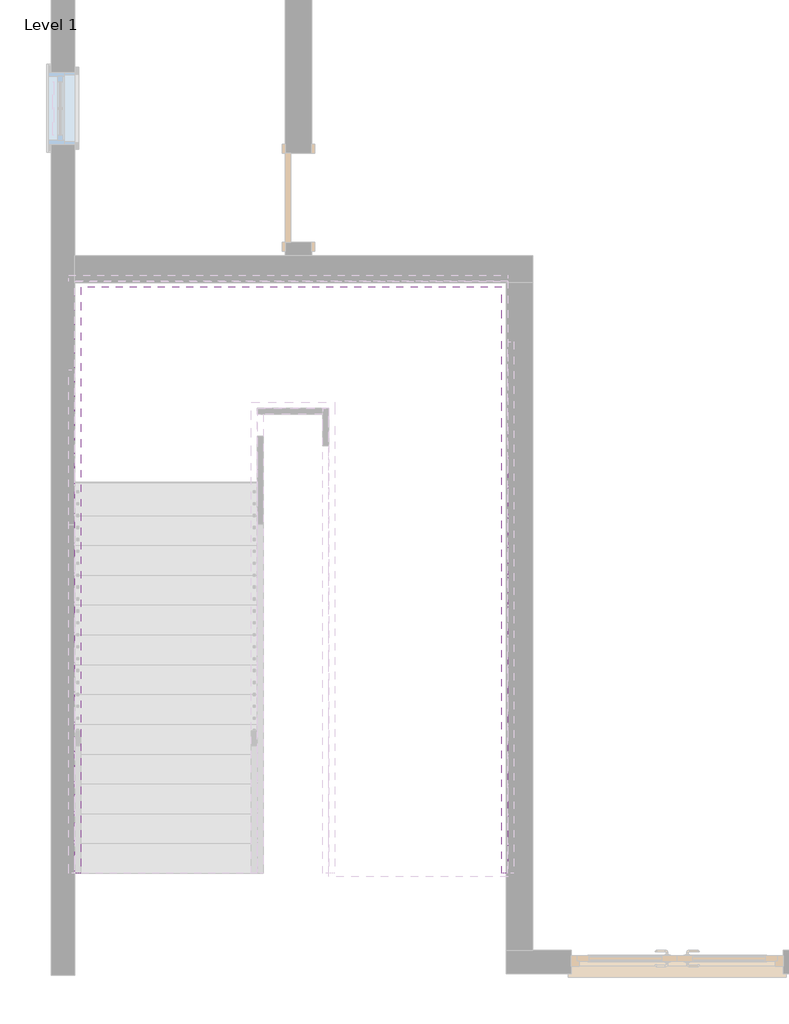
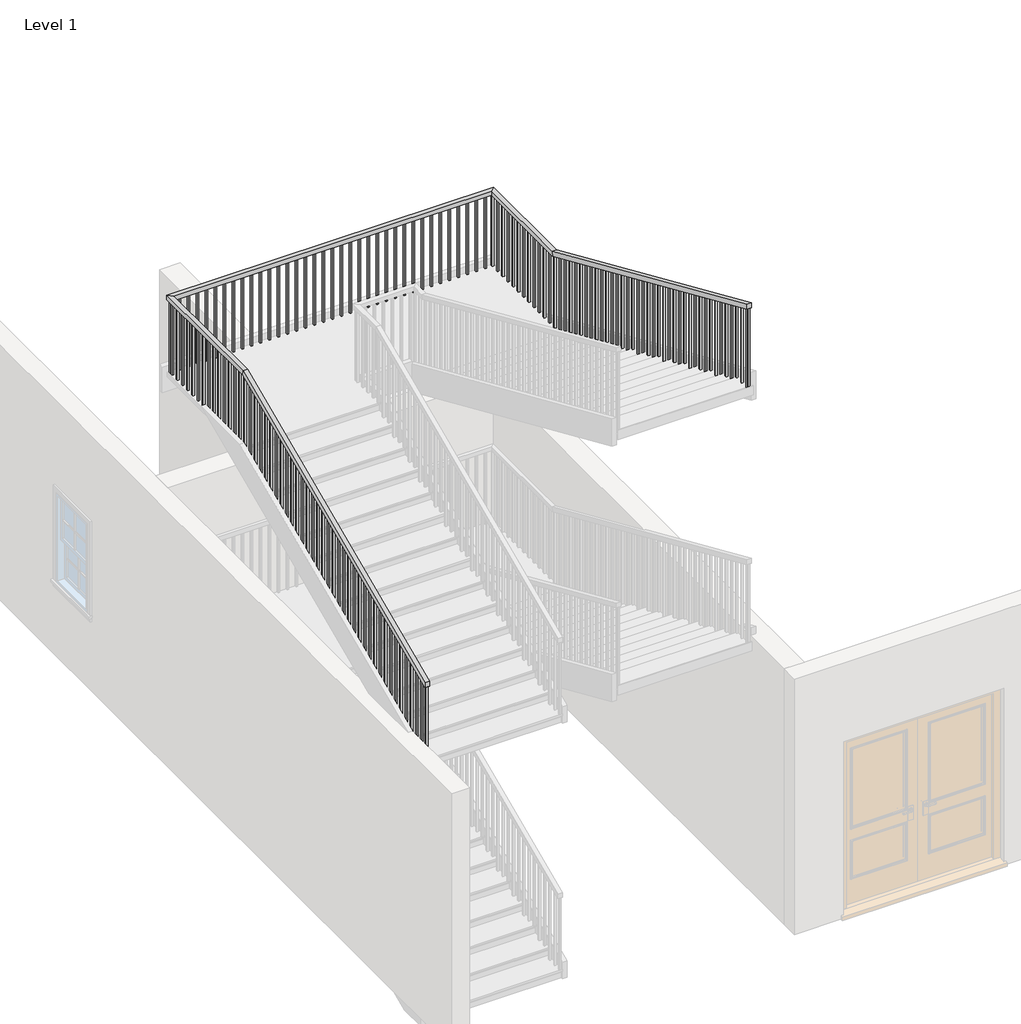
# One storey, part 5 of 6: 1 railing.
"""IFC4 building model written with IfcOpenShell, lengths in millimetres."""

from ifc_helpers import new_model, si_unit, frame, origin, place, context, project, spatial, polyline, outline, extrude, faceted_brep, element, save

model = new_model("IFC4")

# Units and contexts
model_context = context("Model", 3, world=origin())
ifc_project = project(units=[si_unit("LENGTHUNIT", "METRE", prefix="MILLI")], contexts=[model_context])

# Site, building, storey
site = spatial("IfcSite", under=ifc_project)
building = spatial("IfcBuilding", under=site)
storey = spatial("IfcBuildingStorey", under=building, Name="Level 1", Elevation=0.0)

# Railing
placement = place(None, origin())
element("IfcRailing", 1, ObjectType="Handrail - Rectangular", at=placement, inside=storey, context=model_context, shape_type="SolidModel", body=[
    faceted_brep([(-7554.4415084, -6973.0610642, 3769.36), (-7554.4415084, -6973.0610642, 3713.8599828), (-7503.6415084, -6973.0610642, 3713.8599828), (-7503.6415084, -6973.0610642, 3769.36), (-7554.4415084, -3417.0610642, 5334.0), (-7554.4415084, -3406.3792071, 5283.2), (-7503.6415084, -3406.3792071, 5283.2), (-7503.6415084, -3417.0610642, 5334.0), (-7554.4415084, -1928.4217109, 5334.0), (-7554.4415084, -1928.4217109, 5283.2), (-7503.6415084, -1979.2217109, 5283.2), (-7503.6415084, -1979.2217109, 5334.0), (-3866.3290366, -1928.4217109, 5334.0), (-3866.3290366, -1928.4217109, 5283.2), (-3917.1290366, -1979.2217109, 5283.2), (-3917.1290366, -1979.2217109, 5334.0), (-3866.3290366, -3163.0610642, 5334.0), (-3866.3290366, -3173.7429214, 5283.2), (-3917.1290366, -3173.7429214, 5283.2), (-3917.1290366, -3163.0610642, 5334.0), (-3866.3290366, -6973.0610642, 7010.4), (-3917.1290366, -6973.0610642, 7010.4), (-3917.1290366, -6973.0610642, 6954.8999828), (-3866.3290366, -6973.0610642, 6954.8999828)], [[[0, 1, 2, 3]], [[1, 0, 4, 5]], [[2, 1, 5, 6]], [[3, 2, 6, 7]], [[0, 3, 7, 4]], [[5, 4, 8, 9]], [[6, 5, 9, 10]], [[7, 6, 10, 11]], [[4, 7, 11, 8]], [[9, 8, 12, 13]], [[10, 9, 13, 14]], [[11, 10, 14, 15]], [[8, 11, 15, 12]], [[13, 12, 16, 17]], [[14, 13, 17, 18]], [[15, 14, 18, 19]], [[12, 15, 19, 16]], [[20, 21, 22, 23]], [[17, 16, 20, 23]], [[18, 17, 23, 22]], [[19, 18, 22, 21]], [[16, 19, 21, 20]]]),
    extrude(outline(polyline([(-6922.6967109, 6932.7396674), (-6922.6967109, 5984.24), (-6941.7467109, 5984.24), (-6941.7467109, 6941.1216674), (-6922.6967109, 6932.7396674)])), frame((-3901.2540366, 0.0, 0.0), z_axis=(1.0, 0.0, 0.0), x_axis=(0.0, 1.0, 0.0)), (0.0, 0.0, 1.0), 19.05),
    extrude(outline(polyline([(-6821.0967109, 6888.0356674), (-6821.0967109, 5984.24), (-6840.1467109, 5984.24), (-6840.1467109, 6896.4176674), (-6821.0967109, 6888.0356674)])), frame((-3901.2540366, 0.0, 0.0), z_axis=(1.0, 0.0, 0.0), x_axis=(0.0, 1.0, 0.0)), (0.0, 0.0, 1.0), 19.05),
    extrude(outline(polyline([(-6719.4967109, 6843.3316674), (-6719.4967109, 5984.24), (-6738.5467109, 5984.24), (-6738.5467109, 6851.7136674), (-6719.4967109, 6843.3316674)])), frame((-3901.2540366, 0.0, 0.0), z_axis=(1.0, 0.0, 0.0), x_axis=(0.0, 1.0, 0.0)), (0.0, 0.0, 1.0), 19.05),
    extrude(outline(polyline([(-6617.8967109, 6798.6276674), (-6617.8967109, 5872.48), (-6636.9467109, 5872.48), (-6636.9467109, 6807.0096674), (-6617.8967109, 6798.6276674)])), frame((-3901.2540366, 0.0, 0.0), z_axis=(1.0, 0.0, 0.0), x_axis=(0.0, 1.0, 0.0)), (0.0, 0.0, 1.0), 19.05),
    extrude(outline(polyline([(-6516.2967109, 6753.9236674), (-6516.2967109, 5872.48), (-6535.3467109, 5872.48), (-6535.3467109, 6762.3056674), (-6516.2967109, 6753.9236674)])), frame((-3901.2540366, 0.0, 0.0), z_axis=(1.0, 0.0, 0.0), x_axis=(0.0, 1.0, 0.0)), (0.0, 0.0, 1.0), 19.05),
    extrude(outline(polyline([(-6414.6967109, 6709.2196674), (-6414.6967109, 5760.72), (-6433.7467109, 5760.72), (-6433.7467109, 6717.6016674), (-6414.6967109, 6709.2196674)])), frame((-3901.2540366, 0.0, 0.0), z_axis=(1.0, 0.0, 0.0), x_axis=(0.0, 1.0, 0.0)), (0.0, 0.0, 1.0), 19.05),
    extrude(outline(polyline([(-6313.0967109, 6664.5156674), (-6313.0967109, 5760.72), (-6332.1467109, 5760.72), (-6332.1467109, 6672.8976674), (-6313.0967109, 6664.5156674)])), frame((-3901.2540366, 0.0, 0.0), z_axis=(1.0, 0.0, 0.0), x_axis=(0.0, 1.0, 0.0)), (0.0, 0.0, 1.0), 19.05),
    extrude(outline(polyline([(-6211.4967109, 6619.8116674), (-6211.4967109, 5760.72), (-6230.5467109, 5760.72), (-6230.5467109, 6628.1936674), (-6211.4967109, 6619.8116674)])), frame((-3901.2540366, 0.0, 0.0), z_axis=(1.0, 0.0, 0.0), x_axis=(0.0, 1.0, 0.0)), (0.0, 0.0, 1.0), 19.05),
    extrude(outline(polyline([(-6109.8967109, 6575.1076674), (-6109.8967109, 5648.96), (-6128.9467109, 5648.96), (-6128.9467109, 6583.4896674), (-6109.8967109, 6575.1076674)])), frame((-3901.2540366, 0.0, 0.0), z_axis=(1.0, 0.0, 0.0), x_axis=(0.0, 1.0, 0.0)), (0.0, 0.0, 1.0), 19.05),
    extrude(outline(polyline([(-6008.2967109, 6530.4036674), (-6008.2967109, 5648.96), (-6027.3467109, 5648.96), (-6027.3467109, 6538.7856674), (-6008.2967109, 6530.4036674)])), frame((-3901.2540366, 0.0, 0.0), z_axis=(1.0, 0.0, 0.0), x_axis=(0.0, 1.0, 0.0)), (0.0, 0.0, 1.0), 19.05),
    extrude(outline(polyline([(-5906.6967109, 6485.6996674), (-5906.6967109, 5537.2), (-5925.7467109, 5537.2), (-5925.7467109, 6494.0816674), (-5906.6967109, 6485.6996674)])), frame((-3901.2540366, 0.0, 0.0), z_axis=(1.0, 0.0, 0.0), x_axis=(0.0, 1.0, 0.0)), (0.0, 0.0, 1.0), 19.05),
    extrude(outline(polyline([(-5805.0967109, 6440.9956674), (-5805.0967109, 5537.2), (-5824.1467109, 5537.2), (-5824.1467109, 6449.3776674), (-5805.0967109, 6440.9956674)])), frame((-3901.2540366, 0.0, 0.0), z_axis=(1.0, 0.0, 0.0), x_axis=(0.0, 1.0, 0.0)), (0.0, 0.0, 1.0), 19.05),
    extrude(outline(polyline([(-5703.4967109, 6396.2916674), (-5703.4967109, 5537.2), (-5722.5467109, 5537.2), (-5722.5467109, 6404.6736674), (-5703.4967109, 6396.2916674)])), frame((-3901.2540366, 0.0, 0.0), z_axis=(1.0, 0.0, 0.0), x_axis=(0.0, 1.0, 0.0)), (0.0, 0.0, 1.0), 19.05),
    extrude(outline(polyline([(-5601.8967109, 6351.5876674), (-5601.8967109, 5425.44), (-5620.9467109, 5425.44), (-5620.9467109, 6359.9696674), (-5601.8967109, 6351.5876674)])), frame((-3901.2540366, 0.0, 0.0), z_axis=(1.0, 0.0, 0.0), x_axis=(0.0, 1.0, 0.0)), (0.0, 0.0, 1.0), 19.05),
    extrude(outline(polyline([(-5500.2967109, 6306.8836674), (-5500.2967109, 5425.44), (-5519.3467109, 5425.44), (-5519.3467109, 6315.2656674), (-5500.2967109, 6306.8836674)])), frame((-3901.2540366, 0.0, 0.0), z_axis=(1.0, 0.0, 0.0), x_axis=(0.0, 1.0, 0.0)), (0.0, 0.0, 1.0), 19.05),
    extrude(outline(polyline([(-5398.6967109, 6262.1796674), (-5398.6967109, 5313.68), (-5417.7467109, 5313.68), (-5417.7467109, 6270.5616674), (-5398.6967109, 6262.1796674)])), frame((-3901.2540366, 0.0, 0.0), z_axis=(1.0, 0.0, 0.0), x_axis=(0.0, 1.0, 0.0)), (0.0, 0.0, 1.0), 19.05),
    extrude(outline(polyline([(-5297.0967109, 6217.4756674), (-5297.0967109, 5313.68), (-5316.1467109, 5313.68), (-5316.1467109, 6225.8576674), (-5297.0967109, 6217.4756674)])), frame((-3901.2540366, 0.0, 0.0), z_axis=(1.0, 0.0, 0.0), x_axis=(0.0, 1.0, 0.0)), (0.0, 0.0, 1.0), 19.05),
    extrude(outline(polyline([(-5195.4967109, 6172.7716674), (-5195.4967109, 5313.68), (-5214.5467109, 5313.68), (-5214.5467109, 6181.1536674), (-5195.4967109, 6172.7716674)])), frame((-3901.2540366, 0.0, 0.0), z_axis=(1.0, 0.0, 0.0), x_axis=(0.0, 1.0, 0.0)), (0.0, 0.0, 1.0), 19.05),
    extrude(outline(polyline([(-5093.8967109, 6128.0676674), (-5093.8967109, 5201.92), (-5112.9467109, 5201.92), (-5112.9467109, 6136.4496674), (-5093.8967109, 6128.0676674)])), frame((-3901.2540366, 0.0, 0.0), z_axis=(1.0, 0.0, 0.0), x_axis=(0.0, 1.0, 0.0)), (0.0, 0.0, 1.0), 19.05),
    extrude(outline(polyline([(-4992.2967109, 6083.3636674), (-4992.2967109, 5201.92), (-5011.3467109, 5201.92), (-5011.3467109, 6091.7456674), (-4992.2967109, 6083.3636674)])), frame((-3901.2540366, 0.0, 0.0), z_axis=(1.0, 0.0, 0.0), x_axis=(0.0, 1.0, 0.0)), (0.0, 0.0, 1.0), 19.05),
    extrude(outline(polyline([(-4890.6967109, 6038.6596674), (-4890.6967109, 5090.16), (-4909.7467109, 5090.16), (-4909.7467109, 6047.0416674), (-4890.6967109, 6038.6596674)])), frame((-3901.2540366, 0.0, 0.0), z_axis=(1.0, 0.0, 0.0), x_axis=(0.0, 1.0, 0.0)), (0.0, 0.0, 1.0), 19.05),
    extrude(outline(polyline([(-4789.0967109, 5993.9556674), (-4789.0967109, 5090.16), (-4808.1467109, 5090.16), (-4808.1467109, 6002.3376674), (-4789.0967109, 5993.9556674)])), frame((-3901.2540366, 0.0, 0.0), z_axis=(1.0, 0.0, 0.0), x_axis=(0.0, 1.0, 0.0)), (0.0, 0.0, 1.0), 19.05),
    extrude(outline(polyline([(-4687.4967109, 5949.2516674), (-4687.4967109, 5090.16), (-4706.5467109, 5090.16), (-4706.5467109, 5957.6336674), (-4687.4967109, 5949.2516674)])), frame((-3901.2540366, 0.0, 0.0), z_axis=(1.0, 0.0, 0.0), x_axis=(0.0, 1.0, 0.0)), (0.0, 0.0, 1.0), 19.05),
    extrude(outline(polyline([(-4585.8967109, 5904.5476674), (-4585.8967109, 4978.4), (-4604.9467109, 4978.4), (-4604.9467109, 5912.9296674), (-4585.8967109, 5904.5476674)])), frame((-3901.2540366, 0.0, 0.0), z_axis=(1.0, 0.0, 0.0), x_axis=(0.0, 1.0, 0.0)), (0.0, 0.0, 1.0), 19.05),
    extrude(outline(polyline([(-4484.2967109, 5859.8436674), (-4484.2967109, 4978.4), (-4503.3467109, 4978.4), (-4503.3467109, 5868.2256674), (-4484.2967109, 5859.8436674)])), frame((-3901.2540366, 0.0, 0.0), z_axis=(1.0, 0.0, 0.0), x_axis=(0.0, 1.0, 0.0)), (0.0, 0.0, 1.0), 19.05),
    extrude(outline(polyline([(-4382.6967109, 5815.1396674), (-4382.6967109, 4866.64), (-4401.7467109, 4866.64), (-4401.7467109, 5823.5216674), (-4382.6967109, 5815.1396674)])), frame((-3901.2540366, 0.0, 0.0), z_axis=(1.0, 0.0, 0.0), x_axis=(0.0, 1.0, 0.0)), (0.0, 0.0, 1.0), 19.05),
    extrude(outline(polyline([(-4281.0967109, 5770.4356674), (-4281.0967109, 4866.64), (-4300.1467109, 4866.64), (-4300.1467109, 5778.8176674), (-4281.0967109, 5770.4356674)])), frame((-3901.2540366, 0.0, 0.0), z_axis=(1.0, 0.0, 0.0), x_axis=(0.0, 1.0, 0.0)), (0.0, 0.0, 1.0), 19.05),
    extrude(outline(polyline([(-4179.4967109, 5725.7316674), (-4179.4967109, 4866.64), (-4198.5467109, 4866.64), (-4198.5467109, 5734.1136674), (-4179.4967109, 5725.7316674)])), frame((-3901.2540366, 0.0, 0.0), z_axis=(1.0, 0.0, 0.0), x_axis=(0.0, 1.0, 0.0)), (0.0, 0.0, 1.0), 19.05),
    extrude(outline(polyline([(-4077.8967109, 5681.0276674), (-4077.8967109, 4754.88), (-4096.9467109, 4754.88), (-4096.9467109, 5689.4096674), (-4077.8967109, 5681.0276674)])), frame((-3901.2540366, 0.0, 0.0), z_axis=(1.0, 0.0, 0.0), x_axis=(0.0, 1.0, 0.0)), (0.0, 0.0, 1.0), 19.05),
    extrude(outline(polyline([(-3976.2967109, 5636.3236674), (-3976.2967109, 4754.88), (-3995.3467109, 4754.88), (-3995.3467109, 5644.7056674), (-3976.2967109, 5636.3236674)])), frame((-3901.2540366, 0.0, 0.0), z_axis=(1.0, 0.0, 0.0), x_axis=(0.0, 1.0, 0.0)), (0.0, 0.0, 1.0), 19.05),
    extrude(outline(polyline([(-3874.6967109, 5591.6196674), (-3874.6967109, 4643.12), (-3893.7467109, 4643.12), (-3893.7467109, 5600.0016674), (-3874.6967109, 5591.6196674)])), frame((-3901.2540366, 0.0, 0.0), z_axis=(1.0, 0.0, 0.0), x_axis=(0.0, 1.0, 0.0)), (0.0, 0.0, 1.0), 19.05),
    extrude(outline(polyline([(-3773.0967109, 5546.9156674), (-3773.0967109, 4643.12), (-3792.1467109, 4643.12), (-3792.1467109, 5555.2976674), (-3773.0967109, 5546.9156674)])), frame((-3901.2540366, 0.0, 0.0), z_axis=(1.0, 0.0, 0.0), x_axis=(0.0, 1.0, 0.0)), (0.0, 0.0, 1.0), 19.05),
    extrude(outline(polyline([(-3671.4967109, 5502.2116674), (-3671.4967109, 4643.12), (-3690.5467109, 4643.12), (-3690.5467109, 5510.5936674), (-3671.4967109, 5502.2116674)])), frame((-3901.2540366, 0.0, 0.0), z_axis=(1.0, 0.0, 0.0), x_axis=(0.0, 1.0, 0.0)), (0.0, 0.0, 1.0), 19.05),
    extrude(outline(polyline([(-3569.8967109, 5457.5076674), (-3569.8967109, 4531.36), (-3588.9467109, 4531.36), (-3588.9467109, 5465.8896674), (-3569.8967109, 5457.5076674)])), frame((-3901.2540366, 0.0, 0.0), z_axis=(1.0, 0.0, 0.0), x_axis=(0.0, 1.0, 0.0)), (0.0, 0.0, 1.0), 19.05),
    extrude(outline(polyline([(-3468.2967109, 5412.8036674), (-3468.2967109, 4531.36), (-3487.3467109, 4531.36), (-3487.3467109, 5421.1856674), (-3468.2967109, 5412.8036674)])), frame((-3901.2540366, 0.0, 0.0), z_axis=(1.0, 0.0, 0.0), x_axis=(0.0, 1.0, 0.0)), (0.0, 0.0, 1.0), 19.05),
    extrude(outline(polyline([(-3366.6967109, 5368.0996674), (-3366.6967109, 4419.6), (-3385.7467109, 4419.6), (-3385.7467109, 5376.4816674), (-3366.6967109, 5368.0996674)])), frame((-3901.2540366, 0.0, 0.0), z_axis=(1.0, 0.0, 0.0), x_axis=(0.0, 1.0, 0.0)), (0.0, 0.0, 1.0), 19.05),
    extrude(outline(polyline([(-3265.0967109, 5323.3956674), (-3265.0967109, 4419.6), (-3284.1467109, 4419.6), (-3284.1467109, 5331.7776674), (-3265.0967109, 5323.3956674)])), frame((-3901.2540366, 0.0, 0.0), z_axis=(1.0, 0.0, 0.0), x_axis=(0.0, 1.0, 0.0)), (0.0, 0.0, 1.0), 19.05),
    extrude(outline(polyline([(-3163.4967109, 5278.6916674), (-3163.4967109, 4419.6), (-3182.5467109, 4419.6), (-3182.5467109, 5287.0736674), (-3163.4967109, 5278.6916674)])), frame((-3901.2540366, 0.0, 0.0), z_axis=(1.0, 0.0, 0.0), x_axis=(0.0, 1.0, 0.0)), (0.0, 0.0, 1.0), 19.05),
    extrude(outline(polyline([(-3882.2040366, -3061.8967109), (-3882.2040366, -3080.9467109), (-3901.2540366, -3080.9467109), (-3901.2540366, -3061.8967109), (-3882.2040366, -3061.8967109)])), frame((0.0, 0.0, 4419.6), z_axis=(0.0, 0.0, 1.0), x_axis=(1.0, 0.0, 0.0)), (0.0, 0.0, 1.0), 863.6),
    extrude(outline(polyline([(-3882.2040366, -2960.2967109), (-3882.2040366, -2979.3467109), (-3901.2540366, -2979.3467109), (-3901.2540366, -2960.2967109), (-3882.2040366, -2960.2967109)])), frame((0.0, 0.0, 4419.6), z_axis=(0.0, 0.0, 1.0), x_axis=(1.0, 0.0, 0.0)), (0.0, 0.0, 1.0), 863.6),
    extrude(outline(polyline([(-3882.2040366, -2858.6967109), (-3882.2040366, -2877.7467109), (-3901.2540366, -2877.7467109), (-3901.2540366, -2858.6967109), (-3882.2040366, -2858.6967109)])), frame((0.0, 0.0, 4419.6), z_axis=(0.0, 0.0, 1.0), x_axis=(1.0, 0.0, 0.0)), (0.0, 0.0, 1.0), 863.6),
    extrude(outline(polyline([(-3882.2040366, -2757.0967109), (-3882.2040366, -2776.1467109), (-3901.2540366, -2776.1467109), (-3901.2540366, -2757.0967109), (-3882.2040366, -2757.0967109)])), frame((0.0, 0.0, 4419.6), z_axis=(0.0, 0.0, 1.0), x_axis=(1.0, 0.0, 0.0)), (0.0, 0.0, 1.0), 863.6),
    extrude(outline(polyline([(-3882.2040366, -2655.4967109), (-3882.2040366, -2674.5467109), (-3901.2540366, -2674.5467109), (-3901.2540366, -2655.4967109), (-3882.2040366, -2655.4967109)])), frame((0.0, 0.0, 4419.6), z_axis=(0.0, 0.0, 1.0), x_axis=(1.0, 0.0, 0.0)), (0.0, 0.0, 1.0), 863.6),
    extrude(outline(polyline([(-3882.2040366, -2553.8967109), (-3882.2040366, -2572.9467109), (-3901.2540366, -2572.9467109), (-3901.2540366, -2553.8967109), (-3882.2040366, -2553.8967109)])), frame((0.0, 0.0, 4419.6), z_axis=(0.0, 0.0, 1.0), x_axis=(1.0, 0.0, 0.0)), (0.0, 0.0, 1.0), 863.6),
    extrude(outline(polyline([(-3882.2040366, -2452.2967109), (-3882.2040366, -2471.3467109), (-3901.2540366, -2471.3467109), (-3901.2540366, -2452.2967109), (-3882.2040366, -2452.2967109)])), frame((0.0, 0.0, 4419.6), z_axis=(0.0, 0.0, 1.0), x_axis=(1.0, 0.0, 0.0)), (0.0, 0.0, 1.0), 863.6),
    extrude(outline(polyline([(-3882.2040366, -2350.6967109), (-3882.2040366, -2369.7467109), (-3901.2540366, -2369.7467109), (-3901.2540366, -2350.6967109), (-3882.2040366, -2350.6967109)])), frame((0.0, 0.0, 4419.6), z_axis=(0.0, 0.0, 1.0), x_axis=(1.0, 0.0, 0.0)), (0.0, 0.0, 1.0), 863.6),
    extrude(outline(polyline([(-3882.2040366, -2249.0967109), (-3882.2040366, -2268.1467109), (-3901.2540366, -2268.1467109), (-3901.2540366, -2249.0967109), (-3882.2040366, -2249.0967109)])), frame((0.0, 0.0, 4419.6), z_axis=(0.0, 0.0, 1.0), x_axis=(1.0, 0.0, 0.0)), (0.0, 0.0, 1.0), 863.6),
    extrude(outline(polyline([(-3882.2040366, -2147.4967109), (-3882.2040366, -2166.5467109), (-3901.2540366, -2166.5467109), (-3901.2540366, -2147.4967109), (-3882.2040366, -2147.4967109)])), frame((0.0, 0.0, 4419.6), z_axis=(0.0, 0.0, 1.0), x_axis=(1.0, 0.0, 0.0)), (0.0, 0.0, 1.0), 863.6),
    extrude(outline(polyline([(-3882.2040366, -2045.8967109), (-3882.2040366, -2064.9467109), (-3901.2540366, -2064.9467109), (-3901.2540366, -2045.8967109), (-3882.2040366, -2045.8967109)])), frame((0.0, 0.0, 4419.6), z_axis=(0.0, 0.0, 1.0), x_axis=(1.0, 0.0, 0.0)), (0.0, 0.0, 1.0), 863.6),
    extrude(outline(polyline([(-3982.5665084, -1944.2967109), (-3963.5165084, -1944.2967109), (-3963.5165084, -1963.3467109), (-3982.5665084, -1963.3467109), (-3982.5665084, -1944.2967109)])), frame((0.0, 0.0, 4419.6), z_axis=(0.0, 0.0, 1.0), x_axis=(1.0, 0.0, 0.0)), (0.0, 0.0, 1.0), 863.6),
    extrude(outline(polyline([(-4084.1665084, -1944.2967109), (-4065.1165084, -1944.2967109), (-4065.1165084, -1963.3467109), (-4084.1665084, -1963.3467109), (-4084.1665084, -1944.2967109)])), frame((0.0, 0.0, 4419.6), z_axis=(0.0, 0.0, 1.0), x_axis=(1.0, 0.0, 0.0)), (0.0, 0.0, 1.0), 863.6),
    extrude(outline(polyline([(-4185.7665084, -1944.2967109), (-4166.7165084, -1944.2967109), (-4166.7165084, -1963.3467109), (-4185.7665084, -1963.3467109), (-4185.7665084, -1944.2967109)])), frame((0.0, 0.0, 4419.6), z_axis=(0.0, 0.0, 1.0), x_axis=(1.0, 0.0, 0.0)), (0.0, 0.0, 1.0), 863.6),
    extrude(outline(polyline([(-4287.3665084, -1944.2967109), (-4268.3165084, -1944.2967109), (-4268.3165084, -1963.3467109), (-4287.3665084, -1963.3467109), (-4287.3665084, -1944.2967109)])), frame((0.0, 0.0, 4419.6), z_axis=(0.0, 0.0, 1.0), x_axis=(1.0, 0.0, 0.0)), (0.0, 0.0, 1.0), 863.6),
    extrude(outline(polyline([(-4388.9665084, -1944.2967109), (-4369.9165084, -1944.2967109), (-4369.9165084, -1963.3467109), (-4388.9665084, -1963.3467109), (-4388.9665084, -1944.2967109)])), frame((0.0, 0.0, 4419.6), z_axis=(0.0, 0.0, 1.0), x_axis=(1.0, 0.0, 0.0)), (0.0, 0.0, 1.0), 863.6),
    extrude(outline(polyline([(-4490.5665084, -1944.2967109), (-4471.5165084, -1944.2967109), (-4471.5165084, -1963.3467109), (-4490.5665084, -1963.3467109), (-4490.5665084, -1944.2967109)])), frame((0.0, 0.0, 4419.6), z_axis=(0.0, 0.0, 1.0), x_axis=(1.0, 0.0, 0.0)), (0.0, 0.0, 1.0), 863.6),
    extrude(outline(polyline([(-4592.1665084, -1944.2967109), (-4573.1165084, -1944.2967109), (-4573.1165084, -1963.3467109), (-4592.1665084, -1963.3467109), (-4592.1665084, -1944.2967109)])), frame((0.0, 0.0, 4419.6), z_axis=(0.0, 0.0, 1.0), x_axis=(1.0, 0.0, 0.0)), (0.0, 0.0, 1.0), 863.6),
    extrude(outline(polyline([(-4693.7665084, -1944.2967109), (-4674.7165084, -1944.2967109), (-4674.7165084, -1963.3467109), (-4693.7665084, -1963.3467109), (-4693.7665084, -1944.2967109)])), frame((0.0, 0.0, 4419.6), z_axis=(0.0, 0.0, 1.0), x_axis=(1.0, 0.0, 0.0)), (0.0, 0.0, 1.0), 863.6),
    extrude(outline(polyline([(-4795.3665084, -1944.2967109), (-4776.3165084, -1944.2967109), (-4776.3165084, -1963.3467109), (-4795.3665084, -1963.3467109), (-4795.3665084, -1944.2967109)])), frame((0.0, 0.0, 4419.6), z_axis=(0.0, 0.0, 1.0), x_axis=(1.0, 0.0, 0.0)), (0.0, 0.0, 1.0), 863.6),
    extrude(outline(polyline([(-4896.9665084, -1944.2967109), (-4877.9165084, -1944.2967109), (-4877.9165084, -1963.3467109), (-4896.9665084, -1963.3467109), (-4896.9665084, -1944.2967109)])), frame((0.0, 0.0, 4419.6), z_axis=(0.0, 0.0, 1.0), x_axis=(1.0, 0.0, 0.0)), (0.0, 0.0, 1.0), 863.6),
    extrude(outline(polyline([(-4998.5665084, -1944.2967109), (-4979.5165084, -1944.2967109), (-4979.5165084, -1963.3467109), (-4998.5665084, -1963.3467109), (-4998.5665084, -1944.2967109)])), frame((0.0, 0.0, 4419.6), z_axis=(0.0, 0.0, 1.0), x_axis=(1.0, 0.0, 0.0)), (0.0, 0.0, 1.0), 863.6),
    extrude(outline(polyline([(-5100.1665084, -1944.2967109), (-5081.1165084, -1944.2967109), (-5081.1165084, -1963.3467109), (-5100.1665084, -1963.3467109), (-5100.1665084, -1944.2967109)])), frame((0.0, 0.0, 4419.6), z_axis=(0.0, 0.0, 1.0), x_axis=(1.0, 0.0, 0.0)), (0.0, 0.0, 1.0), 863.6),
    extrude(outline(polyline([(-5201.7665084, -1944.2967109), (-5182.7165084, -1944.2967109), (-5182.7165084, -1963.3467109), (-5201.7665084, -1963.3467109), (-5201.7665084, -1944.2967109)])), frame((0.0, 0.0, 4419.6), z_axis=(0.0, 0.0, 1.0), x_axis=(1.0, 0.0, 0.0)), (0.0, 0.0, 1.0), 863.6),
    extrude(outline(polyline([(-5303.3665084, -1944.2967109), (-5284.3165084, -1944.2967109), (-5284.3165084, -1963.3467109), (-5303.3665084, -1963.3467109), (-5303.3665084, -1944.2967109)])), frame((0.0, 0.0, 4419.6), z_axis=(0.0, 0.0, 1.0), x_axis=(1.0, 0.0, 0.0)), (0.0, 0.0, 1.0), 863.6),
    extrude(outline(polyline([(-5404.9665084, -1944.2967109), (-5385.9165084, -1944.2967109), (-5385.9165084, -1963.3467109), (-5404.9665084, -1963.3467109), (-5404.9665084, -1944.2967109)])), frame((0.0, 0.0, 4419.6), z_axis=(0.0, 0.0, 1.0), x_axis=(1.0, 0.0, 0.0)), (0.0, 0.0, 1.0), 863.6),
    extrude(outline(polyline([(-5506.5665084, -1944.2967109), (-5487.5165084, -1944.2967109), (-5487.5165084, -1963.3467109), (-5506.5665084, -1963.3467109), (-5506.5665084, -1944.2967109)])), frame((0.0, 0.0, 4419.6), z_axis=(0.0, 0.0, 1.0), x_axis=(1.0, 0.0, 0.0)), (0.0, 0.0, 1.0), 863.6),
    extrude(outline(polyline([(-5608.1665084, -1944.2967109), (-5589.1165084, -1944.2967109), (-5589.1165084, -1963.3467109), (-5608.1665084, -1963.3467109), (-5608.1665084, -1944.2967109)])), frame((0.0, 0.0, 4419.6), z_axis=(0.0, 0.0, 1.0), x_axis=(1.0, 0.0, 0.0)), (0.0, 0.0, 1.0), 863.6),
    extrude(outline(polyline([(-5709.7665084, -1944.2967109), (-5690.7165084, -1944.2967109), (-5690.7165084, -1963.3467109), (-5709.7665084, -1963.3467109), (-5709.7665084, -1944.2967109)])), frame((0.0, 0.0, 4419.6), z_axis=(0.0, 0.0, 1.0), x_axis=(1.0, 0.0, 0.0)), (0.0, 0.0, 1.0), 863.6),
    extrude(outline(polyline([(-5811.3665084, -1944.2967109), (-5792.3165084, -1944.2967109), (-5792.3165084, -1963.3467109), (-5811.3665084, -1963.3467109), (-5811.3665084, -1944.2967109)])), frame((0.0, 0.0, 4419.6), z_axis=(0.0, 0.0, 1.0), x_axis=(1.0, 0.0, 0.0)), (0.0, 0.0, 1.0), 863.6),
    extrude(outline(polyline([(-5912.9665084, -1944.2967109), (-5893.9165084, -1944.2967109), (-5893.9165084, -1963.3467109), (-5912.9665084, -1963.3467109), (-5912.9665084, -1944.2967109)])), frame((0.0, 0.0, 4419.6), z_axis=(0.0, 0.0, 1.0), x_axis=(1.0, 0.0, 0.0)), (0.0, 0.0, 1.0), 863.6),
    extrude(outline(polyline([(-6014.5665084, -1944.2967109), (-5995.5165084, -1944.2967109), (-5995.5165084, -1963.3467109), (-6014.5665084, -1963.3467109), (-6014.5665084, -1944.2967109)])), frame((0.0, 0.0, 4419.6), z_axis=(0.0, 0.0, 1.0), x_axis=(1.0, 0.0, 0.0)), (0.0, 0.0, 1.0), 863.6),
    extrude(outline(polyline([(-6116.1665084, -1944.2967109), (-6097.1165084, -1944.2967109), (-6097.1165084, -1963.3467109), (-6116.1665084, -1963.3467109), (-6116.1665084, -1944.2967109)])), frame((0.0, 0.0, 4419.6), z_axis=(0.0, 0.0, 1.0), x_axis=(1.0, 0.0, 0.0)), (0.0, 0.0, 1.0), 863.6),
    extrude(outline(polyline([(-6217.7665084, -1944.2967109), (-6198.7165084, -1944.2967109), (-6198.7165084, -1963.3467109), (-6217.7665084, -1963.3467109), (-6217.7665084, -1944.2967109)])), frame((0.0, 0.0, 4419.6), z_axis=(0.0, 0.0, 1.0), x_axis=(1.0, 0.0, 0.0)), (0.0, 0.0, 1.0), 863.6),
    extrude(outline(polyline([(-6319.3665084, -1944.2967109), (-6300.3165084, -1944.2967109), (-6300.3165084, -1963.3467109), (-6319.3665084, -1963.3467109), (-6319.3665084, -1944.2967109)])), frame((0.0, 0.0, 4419.6), z_axis=(0.0, 0.0, 1.0), x_axis=(1.0, 0.0, 0.0)), (0.0, 0.0, 1.0), 863.6),
    extrude(outline(polyline([(-6420.9665084, -1944.2967109), (-6401.9165084, -1944.2967109), (-6401.9165084, -1963.3467109), (-6420.9665084, -1963.3467109), (-6420.9665084, -1944.2967109)])), frame((0.0, 0.0, 4419.6), z_axis=(0.0, 0.0, 1.0), x_axis=(1.0, 0.0, 0.0)), (0.0, 0.0, 1.0), 863.6),
    extrude(outline(polyline([(-6522.5665084, -1944.2967109), (-6503.5165084, -1944.2967109), (-6503.5165084, -1963.3467109), (-6522.5665084, -1963.3467109), (-6522.5665084, -1944.2967109)])), frame((0.0, 0.0, 4419.6), z_axis=(0.0, 0.0, 1.0), x_axis=(1.0, 0.0, 0.0)), (0.0, 0.0, 1.0), 863.6),
    extrude(outline(polyline([(-6624.1665084, -1944.2967109), (-6605.1165084, -1944.2967109), (-6605.1165084, -1963.3467109), (-6624.1665084, -1963.3467109), (-6624.1665084, -1944.2967109)])), frame((0.0, 0.0, 4419.6), z_axis=(0.0, 0.0, 1.0), x_axis=(1.0, 0.0, 0.0)), (0.0, 0.0, 1.0), 863.6),
    extrude(outline(polyline([(-6725.7665084, -1944.2967109), (-6706.7165084, -1944.2967109), (-6706.7165084, -1963.3467109), (-6725.7665084, -1963.3467109), (-6725.7665084, -1944.2967109)])), frame((0.0, 0.0, 4419.6), z_axis=(0.0, 0.0, 1.0), x_axis=(1.0, 0.0, 0.0)), (0.0, 0.0, 1.0), 863.6),
    extrude(outline(polyline([(-6827.3665084, -1944.2967109), (-6808.3165084, -1944.2967109), (-6808.3165084, -1963.3467109), (-6827.3665084, -1963.3467109), (-6827.3665084, -1944.2967109)])), frame((0.0, 0.0, 4419.6), z_axis=(0.0, 0.0, 1.0), x_axis=(1.0, 0.0, 0.0)), (0.0, 0.0, 1.0), 863.6),
    extrude(outline(polyline([(-6928.9665084, -1944.2967109), (-6909.9165084, -1944.2967109), (-6909.9165084, -1963.3467109), (-6928.9665084, -1963.3467109), (-6928.9665084, -1944.2967109)])), frame((0.0, 0.0, 4419.6), z_axis=(0.0, 0.0, 1.0), x_axis=(1.0, 0.0, 0.0)), (0.0, 0.0, 1.0), 863.6),
    extrude(outline(polyline([(-7030.5665084, -1944.2967109), (-7011.5165084, -1944.2967109), (-7011.5165084, -1963.3467109), (-7030.5665084, -1963.3467109), (-7030.5665084, -1944.2967109)])), frame((0.0, 0.0, 4419.6), z_axis=(0.0, 0.0, 1.0), x_axis=(1.0, 0.0, 0.0)), (0.0, 0.0, 1.0), 863.6),
    extrude(outline(polyline([(-7132.1665084, -1944.2967109), (-7113.1165084, -1944.2967109), (-7113.1165084, -1963.3467109), (-7132.1665084, -1963.3467109), (-7132.1665084, -1944.2967109)])), frame((0.0, 0.0, 4419.6), z_axis=(0.0, 0.0, 1.0), x_axis=(1.0, 0.0, 0.0)), (0.0, 0.0, 1.0), 863.6),
    extrude(outline(polyline([(-7233.7665084, -1944.2967109), (-7214.7165084, -1944.2967109), (-7214.7165084, -1963.3467109), (-7233.7665084, -1963.3467109), (-7233.7665084, -1944.2967109)])), frame((0.0, 0.0, 4419.6), z_axis=(0.0, 0.0, 1.0), x_axis=(1.0, 0.0, 0.0)), (0.0, 0.0, 1.0), 863.6),
    extrude(outline(polyline([(-7335.3665084, -1944.2967109), (-7316.3165084, -1944.2967109), (-7316.3165084, -1963.3467109), (-7335.3665084, -1963.3467109), (-7335.3665084, -1944.2967109)])), frame((0.0, 0.0, 4419.6), z_axis=(0.0, 0.0, 1.0), x_axis=(1.0, 0.0, 0.0)), (0.0, 0.0, 1.0), 863.6),
    extrude(outline(polyline([(-7436.9665084, -1944.2967109), (-7417.9165084, -1944.2967109), (-7417.9165084, -1963.3467109), (-7436.9665084, -1963.3467109), (-7436.9665084, -1944.2967109)])), frame((0.0, 0.0, 4419.6), z_axis=(0.0, 0.0, 1.0), x_axis=(1.0, 0.0, 0.0)), (0.0, 0.0, 1.0), 863.6),
    extrude(outline(polyline([(-7538.5665084, -2004.1860642), (-7538.5665084, -1985.1360642), (-7519.5165084, -1985.1360642), (-7519.5165084, -2004.1860642), (-7538.5665084, -2004.1860642)])), frame((0.0, 0.0, 4419.6), z_axis=(0.0, 0.0, 1.0), x_axis=(1.0, 0.0, 0.0)), (0.0, 0.0, 1.0), 863.6),
    extrude(outline(polyline([(-7538.5665084, -2105.7860642), (-7538.5665084, -2086.7360642), (-7519.5165084, -2086.7360642), (-7519.5165084, -2105.7860642), (-7538.5665084, -2105.7860642)])), frame((0.0, 0.0, 4419.6), z_axis=(0.0, 0.0, 1.0), x_axis=(1.0, 0.0, 0.0)), (0.0, 0.0, 1.0), 863.6),
    extrude(outline(polyline([(-7538.5665084, -2207.3860642), (-7538.5665084, -2188.3360642), (-7519.5165084, -2188.3360642), (-7519.5165084, -2207.3860642), (-7538.5665084, -2207.3860642)])), frame((0.0, 0.0, 4419.6), z_axis=(0.0, 0.0, 1.0), x_axis=(1.0, 0.0, 0.0)), (0.0, 0.0, 1.0), 863.6),
    extrude(outline(polyline([(-7538.5665084, -2308.9860642), (-7538.5665084, -2289.9360642), (-7519.5165084, -2289.9360642), (-7519.5165084, -2308.9860642), (-7538.5665084, -2308.9860642)])), frame((0.0, 0.0, 4419.6), z_axis=(0.0, 0.0, 1.0), x_axis=(1.0, 0.0, 0.0)), (0.0, 0.0, 1.0), 863.6),
    extrude(outline(polyline([(-7538.5665084, -2410.5860642), (-7538.5665084, -2391.5360642), (-7519.5165084, -2391.5360642), (-7519.5165084, -2410.5860642), (-7538.5665084, -2410.5860642)])), frame((0.0, 0.0, 4419.6), z_axis=(0.0, 0.0, 1.0), x_axis=(1.0, 0.0, 0.0)), (0.0, 0.0, 1.0), 863.6),
    extrude(outline(polyline([(-7538.5665084, -2512.1860642), (-7538.5665084, -2493.1360642), (-7519.5165084, -2493.1360642), (-7519.5165084, -2512.1860642), (-7538.5665084, -2512.1860642)])), frame((0.0, 0.0, 4419.6), z_axis=(0.0, 0.0, 1.0), x_axis=(1.0, 0.0, 0.0)), (0.0, 0.0, 1.0), 863.6),
    extrude(outline(polyline([(-7538.5665084, -2613.7860642), (-7538.5665084, -2594.7360642), (-7519.5165084, -2594.7360642), (-7519.5165084, -2613.7860642), (-7538.5665084, -2613.7860642)])), frame((0.0, 0.0, 4419.6), z_axis=(0.0, 0.0, 1.0), x_axis=(1.0, 0.0, 0.0)), (0.0, 0.0, 1.0), 863.6),
    extrude(outline(polyline([(-7538.5665084, -2715.3860642), (-7538.5665084, -2696.3360642), (-7519.5165084, -2696.3360642), (-7519.5165084, -2715.3860642), (-7538.5665084, -2715.3860642)])), frame((0.0, 0.0, 4419.6), z_axis=(0.0, 0.0, 1.0), x_axis=(1.0, 0.0, 0.0)), (0.0, 0.0, 1.0), 863.6),
    extrude(outline(polyline([(-7538.5665084, -2816.9860642), (-7538.5665084, -2797.9360642), (-7519.5165084, -2797.9360642), (-7519.5165084, -2816.9860642), (-7538.5665084, -2816.9860642)])), frame((0.0, 0.0, 4419.6), z_axis=(0.0, 0.0, 1.0), x_axis=(1.0, 0.0, 0.0)), (0.0, 0.0, 1.0), 863.6),
    extrude(outline(polyline([(-7538.5665084, -2918.5860642), (-7538.5665084, -2899.5360642), (-7519.5165084, -2899.5360642), (-7519.5165084, -2918.5860642), (-7538.5665084, -2918.5860642)])), frame((0.0, 0.0, 4419.6), z_axis=(0.0, 0.0, 1.0), x_axis=(1.0, 0.0, 0.0)), (0.0, 0.0, 1.0), 863.6),
    extrude(outline(polyline([(-7538.5665084, -3020.1860642), (-7538.5665084, -3001.1360642), (-7519.5165084, -3001.1360642), (-7519.5165084, -3020.1860642), (-7538.5665084, -3020.1860642)])), frame((0.0, 0.0, 4419.6), z_axis=(0.0, 0.0, 1.0), x_axis=(1.0, 0.0, 0.0)), (0.0, 0.0, 1.0), 863.6),
    extrude(outline(polyline([(-7538.5665084, -3121.7860642), (-7538.5665084, -3102.7360642), (-7519.5165084, -3102.7360642), (-7519.5165084, -3121.7860642), (-7538.5665084, -3121.7860642)])), frame((0.0, 0.0, 4419.6), z_axis=(0.0, 0.0, 1.0), x_axis=(1.0, 0.0, 0.0)), (0.0, 0.0, 1.0), 863.6),
    extrude(outline(polyline([(-7538.5665084, -3223.3860642), (-7538.5665084, -3204.3360642), (-7519.5165084, -3204.3360642), (-7519.5165084, -3223.3860642), (-7538.5665084, -3223.3860642)])), frame((0.0, 0.0, 4419.6), z_axis=(0.0, 0.0, 1.0), x_axis=(1.0, 0.0, 0.0)), (0.0, 0.0, 1.0), 863.6),
    extrude(outline(polyline([(-7538.5665084, -3324.9860642), (-7538.5665084, -3305.9360642), (-7519.5165084, -3305.9360642), (-7519.5165084, -3324.9860642), (-7538.5665084, -3324.9860642)])), frame((0.0, 0.0, 4419.6), z_axis=(0.0, 0.0, 1.0), x_axis=(1.0, 0.0, 0.0)), (0.0, 0.0, 1.0), 863.6),
    extrude(outline(polyline([(-3407.5360642, 5282.6909828), (-3407.5360642, 4419.6), (-3426.5860642, 4419.6), (-3426.5860642, 5274.3089828), (-3407.5360642, 5282.6909828)])), frame((-7538.5665084, 0.0, 0.0), z_axis=(1.0, 0.0, 0.0), x_axis=(0.0, 1.0, 0.0)), (0.0, 0.0, 1.0), 19.05),
    extrude(outline(polyline([(-3509.1360642, 5237.9869828), (-3509.1360642, 4307.84), (-3528.1860642, 4307.84), (-3528.1860642, 5229.6049828), (-3509.1360642, 5237.9869828)])), frame((-7538.5665084, 0.0, 0.0), z_axis=(1.0, 0.0, 0.0), x_axis=(0.0, 1.0, 0.0)), (0.0, 0.0, 1.0), 19.05),
    extrude(outline(polyline([(-3610.7360642, 5193.2829828), (-3610.7360642, 4307.84), (-3629.7860642, 4307.84), (-3629.7860642, 5184.9009828), (-3610.7360642, 5193.2829828)])), frame((-7538.5665084, 0.0, 0.0), z_axis=(1.0, 0.0, 0.0), x_axis=(0.0, 1.0, 0.0)), (0.0, 0.0, 1.0), 19.05),
    extrude(outline(polyline([(-3712.3360642, 5148.5789828), (-3712.3360642, 4196.08), (-3731.3860642, 4196.08), (-3731.3860642, 5140.1969828), (-3712.3360642, 5148.5789828)])), frame((-7538.5665084, 0.0, 0.0), z_axis=(1.0, 0.0, 0.0), x_axis=(0.0, 1.0, 0.0)), (0.0, 0.0, 1.0), 19.05),
    extrude(outline(polyline([(-3813.9360642, 5103.8749828), (-3813.9360642, 4196.08), (-3832.9860642, 4196.08), (-3832.9860642, 5095.4929828), (-3813.9360642, 5103.8749828)])), frame((-7538.5665084, 0.0, 0.0), z_axis=(1.0, 0.0, 0.0), x_axis=(0.0, 1.0, 0.0)), (0.0, 0.0, 1.0), 19.05),
    extrude(outline(polyline([(-3915.5360642, 5059.1709828), (-3915.5360642, 4196.08), (-3934.5860642, 4196.08), (-3934.5860642, 5050.7889828), (-3915.5360642, 5059.1709828)])), frame((-7538.5665084, 0.0, 0.0), z_axis=(1.0, 0.0, 0.0), x_axis=(0.0, 1.0, 0.0)), (0.0, 0.0, 1.0), 19.05),
    extrude(outline(polyline([(-4017.1360642, 5014.4669828), (-4017.1360642, 4084.32), (-4036.1860642, 4084.32), (-4036.1860642, 5006.0849828), (-4017.1360642, 5014.4669828)])), frame((-7538.5665084, 0.0, 0.0), z_axis=(1.0, 0.0, 0.0), x_axis=(0.0, 1.0, 0.0)), (0.0, 0.0, 1.0), 19.05),
    extrude(outline(polyline([(-4118.7360642, 4969.7629828), (-4118.7360642, 4084.32), (-4137.7860642, 4084.32), (-4137.7860642, 4961.3809828), (-4118.7360642, 4969.7629828)])), frame((-7538.5665084, 0.0, 0.0), z_axis=(1.0, 0.0, 0.0), x_axis=(0.0, 1.0, 0.0)), (0.0, 0.0, 1.0), 19.05),
    extrude(outline(polyline([(-4220.3360642, 4925.0589828), (-4220.3360642, 3972.56), (-4239.3860642, 3972.56), (-4239.3860642, 4916.6769828), (-4220.3360642, 4925.0589828)])), frame((-7538.5665084, 0.0, 0.0), z_axis=(1.0, 0.0, 0.0), x_axis=(0.0, 1.0, 0.0)), (0.0, 0.0, 1.0), 19.05),
    extrude(outline(polyline([(-4321.9360642, 4880.3549828), (-4321.9360642, 3972.56), (-4340.9860642, 3972.56), (-4340.9860642, 4871.9729828), (-4321.9360642, 4880.3549828)])), frame((-7538.5665084, 0.0, 0.0), z_axis=(1.0, 0.0, 0.0), x_axis=(0.0, 1.0, 0.0)), (0.0, 0.0, 1.0), 19.05),
    extrude(outline(polyline([(-4423.5360642, 4835.6509828), (-4423.5360642, 3972.56), (-4442.5860642, 3972.56), (-4442.5860642, 4827.2689828), (-4423.5360642, 4835.6509828)])), frame((-7538.5665084, 0.0, 0.0), z_axis=(1.0, 0.0, 0.0), x_axis=(0.0, 1.0, 0.0)), (0.0, 0.0, 1.0), 19.05),
    extrude(outline(polyline([(-4525.1360642, 4790.9469828), (-4525.1360642, 3860.8), (-4544.1860642, 3860.8), (-4544.1860642, 4782.5649828), (-4525.1360642, 4790.9469828)])), frame((-7538.5665084, 0.0, 0.0), z_axis=(1.0, 0.0, 0.0), x_axis=(0.0, 1.0, 0.0)), (0.0, 0.0, 1.0), 19.05),
    extrude(outline(polyline([(-4626.7360642, 4746.2429828), (-4626.7360642, 3860.8), (-4645.7860642, 3860.8), (-4645.7860642, 4737.8609828), (-4626.7360642, 4746.2429828)])), frame((-7538.5665084, 0.0, 0.0), z_axis=(1.0, 0.0, 0.0), x_axis=(0.0, 1.0, 0.0)), (0.0, 0.0, 1.0), 19.05),
    extrude(outline(polyline([(-4728.3360642, 4701.5389828), (-4728.3360642, 3749.04), (-4747.3860642, 3749.04), (-4747.3860642, 4693.1569828), (-4728.3360642, 4701.5389828)])), frame((-7538.5665084, 0.0, 0.0), z_axis=(1.0, 0.0, 0.0), x_axis=(0.0, 1.0, 0.0)), (0.0, 0.0, 1.0), 19.05),
    extrude(outline(polyline([(-4829.9360642, 4656.8349828), (-4829.9360642, 3749.04), (-4848.9860642, 3749.04), (-4848.9860642, 4648.4529828), (-4829.9360642, 4656.8349828)])), frame((-7538.5665084, 0.0, 0.0), z_axis=(1.0, 0.0, 0.0), x_axis=(0.0, 1.0, 0.0)), (0.0, 0.0, 1.0), 19.05),
    extrude(outline(polyline([(-4931.5360642, 4612.1309828), (-4931.5360642, 3749.04), (-4950.5860642, 3749.04), (-4950.5860642, 4603.7489828), (-4931.5360642, 4612.1309828)])), frame((-7538.5665084, 0.0, 0.0), z_axis=(1.0, 0.0, 0.0), x_axis=(0.0, 1.0, 0.0)), (0.0, 0.0, 1.0), 19.05),
    extrude(outline(polyline([(-5033.1360642, 4567.4269828), (-5033.1360642, 3637.28), (-5052.1860642, 3637.28), (-5052.1860642, 4559.0449828), (-5033.1360642, 4567.4269828)])), frame((-7538.5665084, 0.0, 0.0), z_axis=(1.0, 0.0, 0.0), x_axis=(0.0, 1.0, 0.0)), (0.0, 0.0, 1.0), 19.05),
    extrude(outline(polyline([(-5134.7360642, 4522.7229828), (-5134.7360642, 3637.28), (-5153.7860642, 3637.28), (-5153.7860642, 4514.3409828), (-5134.7360642, 4522.7229828)])), frame((-7538.5665084, 0.0, 0.0), z_axis=(1.0, 0.0, 0.0), x_axis=(0.0, 1.0, 0.0)), (0.0, 0.0, 1.0), 19.05),
    extrude(outline(polyline([(-5236.3360642, 4478.0189828), (-5236.3360642, 3525.52), (-5255.3860642, 3525.52), (-5255.3860642, 4469.6369828), (-5236.3360642, 4478.0189828)])), frame((-7538.5665084, 0.0, 0.0), z_axis=(1.0, 0.0, 0.0), x_axis=(0.0, 1.0, 0.0)), (0.0, 0.0, 1.0), 19.05),
    extrude(outline(polyline([(-5337.9360642, 4433.3149828), (-5337.9360642, 3525.52), (-5356.9860642, 3525.52), (-5356.9860642, 4424.9329828), (-5337.9360642, 4433.3149828)])), frame((-7538.5665084, 0.0, 0.0), z_axis=(1.0, 0.0, 0.0), x_axis=(0.0, 1.0, 0.0)), (0.0, 0.0, 1.0), 19.05),
    extrude(outline(polyline([(-5439.5360642, 4388.6109828), (-5439.5360642, 3525.52), (-5458.5860642, 3525.52), (-5458.5860642, 4380.2289828), (-5439.5360642, 4388.6109828)])), frame((-7538.5665084, 0.0, 0.0), z_axis=(1.0, 0.0, 0.0), x_axis=(0.0, 1.0, 0.0)), (0.0, 0.0, 1.0), 19.05),
    extrude(outline(polyline([(-5541.1360642, 4343.9069828), (-5541.1360642, 3413.76), (-5560.1860642, 3413.76), (-5560.1860642, 4335.5249828), (-5541.1360642, 4343.9069828)])), frame((-7538.5665084, 0.0, 0.0), z_axis=(1.0, 0.0, 0.0), x_axis=(0.0, 1.0, 0.0)), (0.0, 0.0, 1.0), 19.05),
    extrude(outline(polyline([(-5642.7360642, 4299.2029828), (-5642.7360642, 3413.76), (-5661.7860642, 3413.76), (-5661.7860642, 4290.8209828), (-5642.7360642, 4299.2029828)])), frame((-7538.5665084, 0.0, 0.0), z_axis=(1.0, 0.0, 0.0), x_axis=(0.0, 1.0, 0.0)), (0.0, 0.0, 1.0), 19.05),
    extrude(outline(polyline([(-5744.3360642, 4254.4989828), (-5744.3360642, 3302.0), (-5763.3860642, 3302.0), (-5763.3860642, 4246.1169828), (-5744.3360642, 4254.4989828)])), frame((-7538.5665084, 0.0, 0.0), z_axis=(1.0, 0.0, 0.0), x_axis=(0.0, 1.0, 0.0)), (0.0, 0.0, 1.0), 19.05),
    extrude(outline(polyline([(-5845.9360642, 4209.7949828), (-5845.9360642, 3302.0), (-5864.9860642, 3302.0), (-5864.9860642, 4201.4129828), (-5845.9360642, 4209.7949828)])), frame((-7538.5665084, 0.0, 0.0), z_axis=(1.0, 0.0, 0.0), x_axis=(0.0, 1.0, 0.0)), (0.0, 0.0, 1.0), 19.05),
    extrude(outline(polyline([(-5947.5360642, 4165.0909828), (-5947.5360642, 3302.0), (-5966.5860642, 3302.0), (-5966.5860642, 4156.7089828), (-5947.5360642, 4165.0909828)])), frame((-7538.5665084, 0.0, 0.0), z_axis=(1.0, 0.0, 0.0), x_axis=(0.0, 1.0, 0.0)), (0.0, 0.0, 1.0), 19.05),
    extrude(outline(polyline([(-6049.1360642, 4120.3869828), (-6049.1360642, 3190.24), (-6068.1860642, 3190.24), (-6068.1860642, 4112.0049828), (-6049.1360642, 4120.3869828)])), frame((-7538.5665084, 0.0, 0.0), z_axis=(1.0, 0.0, 0.0), x_axis=(0.0, 1.0, 0.0)), (0.0, 0.0, 1.0), 19.05),
    extrude(outline(polyline([(-6150.7360642, 4075.6829828), (-6150.7360642, 3190.24), (-6169.7860642, 3190.24), (-6169.7860642, 4067.3009828), (-6150.7360642, 4075.6829828)])), frame((-7538.5665084, 0.0, 0.0), z_axis=(1.0, 0.0, 0.0), x_axis=(0.0, 1.0, 0.0)), (0.0, 0.0, 1.0), 19.05),
    extrude(outline(polyline([(-6252.3360642, 4030.9789828), (-6252.3360642, 3078.48), (-6271.3860642, 3078.48), (-6271.3860642, 4022.5969828), (-6252.3360642, 4030.9789828)])), frame((-7538.5665084, 0.0, 0.0), z_axis=(1.0, 0.0, 0.0), x_axis=(0.0, 1.0, 0.0)), (0.0, 0.0, 1.0), 19.05),
    extrude(outline(polyline([(-6353.9360642, 3986.2749828), (-6353.9360642, 3078.48), (-6372.9860642, 3078.48), (-6372.9860642, 3977.8929828), (-6353.9360642, 3986.2749828)])), frame((-7538.5665084, 0.0, 0.0), z_axis=(1.0, 0.0, 0.0), x_axis=(0.0, 1.0, 0.0)), (0.0, 0.0, 1.0), 19.05),
    extrude(outline(polyline([(-6455.5360642, 3941.5709828), (-6455.5360642, 3078.48), (-6474.5860642, 3078.48), (-6474.5860642, 3933.1889828), (-6455.5360642, 3941.5709828)])), frame((-7538.5665084, 0.0, 0.0), z_axis=(1.0, 0.0, 0.0), x_axis=(0.0, 1.0, 0.0)), (0.0, 0.0, 1.0), 19.05),
    extrude(outline(polyline([(-6557.1360642, 3896.8669828), (-6557.1360642, 2966.72), (-6576.1860642, 2966.72), (-6576.1860642, 3888.4849828), (-6557.1360642, 3896.8669828)])), frame((-7538.5665084, 0.0, 0.0), z_axis=(1.0, 0.0, 0.0), x_axis=(0.0, 1.0, 0.0)), (0.0, 0.0, 1.0), 19.05),
    extrude(outline(polyline([(-6658.7360642, 3852.1629828), (-6658.7360642, 2966.72), (-6677.7860642, 2966.72), (-6677.7860642, 3843.7809828), (-6658.7360642, 3852.1629828)])), frame((-7538.5665084, 0.0, 0.0), z_axis=(1.0, 0.0, 0.0), x_axis=(0.0, 1.0, 0.0)), (0.0, 0.0, 1.0), 19.05),
    extrude(outline(polyline([(-6760.3360642, 3807.4589828), (-6760.3360642, 2854.96), (-6779.3860642, 2854.96), (-6779.3860642, 3799.0769828), (-6760.3360642, 3807.4589828)])), frame((-7538.5665084, 0.0, 0.0), z_axis=(1.0, 0.0, 0.0), x_axis=(0.0, 1.0, 0.0)), (0.0, 0.0, 1.0), 19.05),
    extrude(outline(polyline([(-6861.9360642, 3762.7549828), (-6861.9360642, 2854.96), (-6880.9860642, 2854.96), (-6880.9860642, 3754.3729828), (-6861.9360642, 3762.7549828)])), frame((-7538.5665084, 0.0, 0.0), z_axis=(1.0, 0.0, 0.0), x_axis=(0.0, 1.0, 0.0)), (0.0, 0.0, 1.0), 19.05),
    extrude(outline(polyline([(-3901.2540366, -1944.2967109), (-3882.2040366, -1944.2967109), (-3882.2040366, -1963.3467109), (-3901.2540366, -1963.3467109), (-3901.2540366, -1944.2967109)])), frame((0.0, 0.0, 4419.6), z_axis=(0.0, 0.0, 1.0), x_axis=(1.0, 0.0, 0.0)), (0.0, 0.0, 1.0), 863.6),
    extrude(outline(polyline([(-7538.5665084, -1963.3467109), (-7538.5665084, -1944.2967109), (-7519.5165084, -1944.2967109), (-7519.5165084, -1963.3467109), (-7538.5665084, -1963.3467109)])), frame((0.0, 0.0, 4419.6), z_axis=(0.0, 0.0, 1.0), x_axis=(1.0, 0.0, 0.0)), (0.0, 0.0, 1.0), 863.6),
    extrude(outline(polyline([(-6954.0110642, 6946.5179828), (-6954.0110642, 5984.24), (-6973.0610642, 5984.24), (-6973.0610642, 6954.8999828), (-6954.0110642, 6946.5179828)])), frame((-3901.2540366, 0.0, 0.0), z_axis=(1.0, 0.0, 0.0), x_axis=(0.0, 1.0, 0.0)), (0.0, 0.0, 1.0), 19.05),
    extrude(outline(polyline([(-6954.0110642, 3722.2419828), (-6954.0110642, 2854.96), (-6973.0610642, 2854.96), (-6973.0610642, 3713.8599828), (-6954.0110642, 3722.2419828)])), frame((-7538.5665084, 0.0, 0.0), z_axis=(1.0, 0.0, 0.0), x_axis=(0.0, 1.0, 0.0)), (0.0, 0.0, 1.0), 19.05),
])

save(model, "model.ifc")

# Revit data of these elements
# Type "Handrail - Rectangular"
#   Assembly Code = "C2010400"
#   built-in parameter 1008612 = 0.0416667 (stored number, unit not read)
#   built-in parameter 1008611 = 0.0416667 (stored number, unit not read)
#   built-in parameter 1008609 = 0.333333 (stored number, unit not read)
#   built-in parameter 1008604 = 0.166667 (stored number, unit not read)
#   built-in parameter 1008603 = 0.166667 (stored number, unit not read)
#   Railing Height = 3' - 0"
#   built-in parameter 1008630 = 2
#   built-in parameter 1008610 = 2
#   built-in parameter 1008618 = Baluster - Square : 3/4"
# Element 1 (IfcRailing, "Handrail - Rectangular")
#   Phase Created = New Construction
